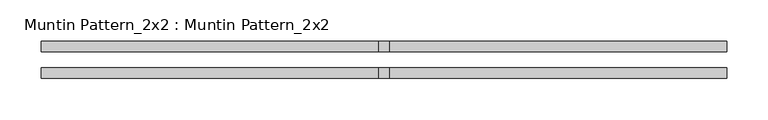
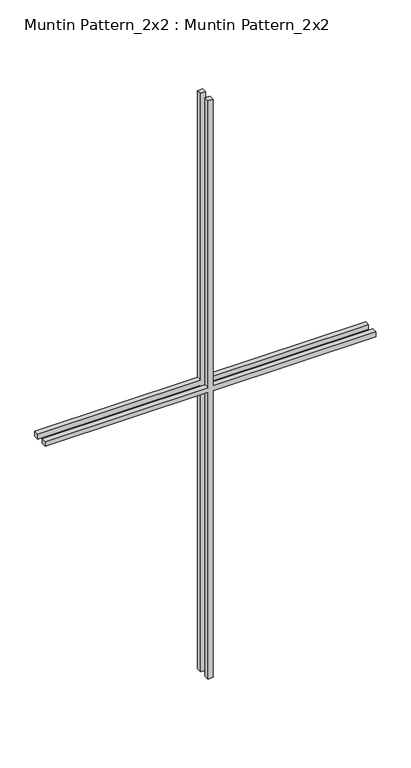
"""IFC4 building model written with IfcOpenShell, lengths in millimetres: proxy geometry, Muntin Pattern_2x2 : Muntin Pattern_2x2."""

from ifc_helpers import new_model, si_unit, frame, origin, place, context, project, spatial, polyline, outline, extrude, source, transform, mapped, element, save


def muntin_pattern_2x2_muntin_pattern_2x2_52b72501(model_context):
    return source(origin(), model_context, "Body", "SweptSolid", [
        extrude(outline(polyline([(771.525, -6.35), (771.525, -414.3375), (758.825, -414.3375), (758.825, -6.35), (0.0, -6.35), (0.0, 6.35), (758.825, 6.35), (758.825, 414.3375), (771.525, 414.3375), (771.525, 6.35), (1530.35, 6.35), (1530.35, -6.35), (771.525, -6.35)])), frame((0.0, 9.525, 0.0), z_axis=(0.0, 1.0, 0.0), x_axis=(0.0, 0.0, 1.0)), (0.0, 0.0, 1.0), 12.7),
        extrude(outline(polyline([(771.525, -6.35), (771.525, -414.3375), (758.825, -414.3375), (758.825, -6.35), (0.0, -6.35), (0.0, 6.35), (758.825, 6.35), (758.825, 414.3375), (771.525, 414.3375), (771.525, 6.35), (1530.35, 6.35), (1530.35, -6.35), (771.525, -6.35)])), frame((0.0, -22.225, 0.0), z_axis=(0.0, 1.0, 0.0), x_axis=(0.0, 0.0, 1.0)), (0.0, 0.0, 1.0), 12.7),
    ])


if __name__ == "__main__":
    model = new_model("IFC4")
    model_context = context("Model", 3, world=origin())
    ifc_project = project(units=[si_unit("LENGTHUNIT", "METRE", prefix="MILLI")], contexts=[model_context])
    site = spatial("IfcSite", under=ifc_project)
    building = spatial("IfcBuilding", under=site)
    placement = place(None, origin())
    muntin_pattern_2x2_muntin_pattern_2x2_shape = muntin_pattern_2x2_muntin_pattern_2x2_52b72501(model_context)
    element("IfcBuildingElementProxy", 1, Name="Muntin Pattern_2x2 : Muntin Pattern_2x2", ObjectType="Muntin Pattern_2x2 : Muntin Pattern_2x2", at=placement, inside=building, context=model_context, shape_type="MappedRepresentation", body=[
        mapped(muntin_pattern_2x2_muntin_pattern_2x2_shape, transform((0.0, 0.0, 0.0), x_axis=(1.0, 0.0, 0.0), y_axis=(0.0, 1.0, 0.0), z_axis=(0.0, 0.0, 1.0))),
    ])
    save(model, "model.ifc")

# Revit data of these elements
# Type "Muntin Pattern_2x2 : Muntin Pattern_2x2"
#   Width [instance default] = 4' - 0"
#   Thickness = 0' - 0 1/2"
#   Height [instance default] = 4' - 0"
#   Distance = 0' - 0 3/4"
#   Interior Material [instance default] = none
#   Exterior Material [instance default] = none
#   Default Elevation = 0
# Element 1 (IfcBuildingElementProxy, "Muntin Pattern_2x2 : Muntin Pattern_2x2")
#   Width = 2' - 8 5/8"
#   Height = 5' - 0 1/4"
#   Interior Material = Wood - Stained
#   Exterior Material = Clad - White
#   Materials on its faces: "Clad - White", "Wood - Stained"
# Materials
#   "Clad - White": class "Wood", colour RGB 242 242 238, transparency 0, Cost = 0
#   "Wood - Stained": class "Wood", colour RGB 224 178 126, transparency 0, Cost = 0
